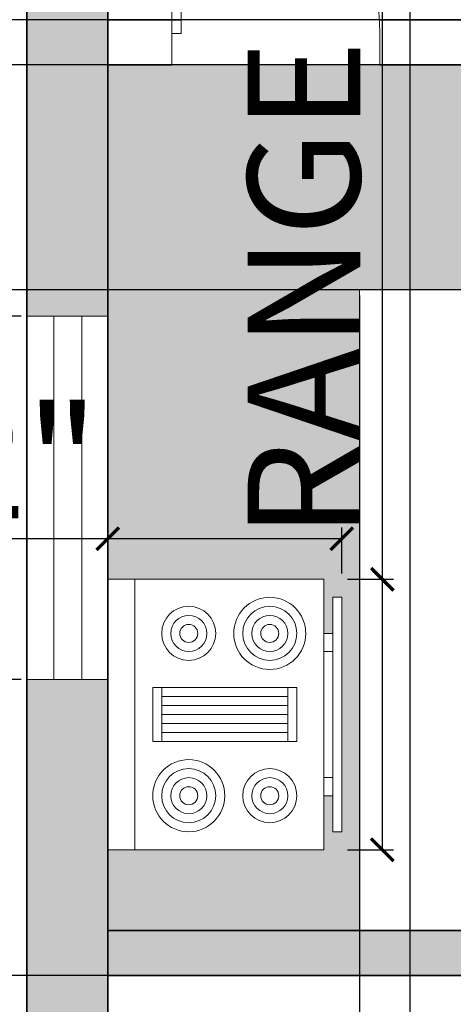
# Model space of a CAD drawing. Units: inches. Extents: x 1763 to 2368, y 1500 to 2097.
# Tile 7 of 24: x 1828 to 1876, y 1877 to 1986. Entities that reach past the tile are written whole.
import ezdxf

# ---------------------------------------------------------------- set-up
doc = ezdxf.new("R2010")
doc.units = ezdxf.units.IN
for name, color, linetype, lineweight in [('A-ANNO-DIMS', 2, 'Continuous', 18), ('A-DOOR', 4, 'Continuous', 18), ('A-EQPM', 9, 'Continuous', 18), ('A-FLOR-CASE', 8, 'Continuous', 18), ('A-WALL', 7, 'Continuous', 35), ('A-WALL-PATT', 7, 'Continuous', 13), ('windows', 1, 'Continuous', 18)]:
    doc.layers.add(name, color=color, linetype=linetype, lineweight=lineweight)
doc.layers.add('A-FLOR-CASE-PATT', color=254, linetype='Continuous', lineweight=13, true_color=0xcecce6)
doc.styles.get("Standard").update_dxf_attribs({"font": 'arial.ttf'})
doc.dimstyles.new('ISO-25', dxfattribs={"dimtxt": 12.5, "dimasz": 2.5, "dimexe": 1.25, "dimexo": 0.625, "dimtad": 1, "dimdec": 0, "dimlunit": 4, "dimtxsty": 'Standard', "dimblk": 'ARCHTICK', "dimcen": 2.5, "dimclrd": 3, "dimclrt": 4, "dimadec": 0, "dimazin": 0, "dimtfac": 1, "dimtdec": 0, "dimtmove": 0, "dimatfit": 3, "dimfxl": 1, "dimarcsym": 0})

# ---------------------------------------------------------------- blocks, each defined once
blk = doc.blocks.new('*U3')
for p, q in [((0, 0), (0, -6)), ((40, 0), (40, -6))]:
    blk.add_line(p, q)
blk.add_lwpolyline([(0, 0), (0, 40), (1.75, 40), (1.75, 0)], close=True)
blk.add_arc((0, 0), 40, 0, 90)
blk = doc.blocks.new('Range-Oven - 30 in top')
for p, q in [((0, -3), (30, -3)), ((12, -6), (18, -6)), ((13, -20), (13, -6)), ((14, -6), (14, -20)), ((15, -20), (15, -6)), ((16, -6), (16, -20)), ((17, -20), (17, -6)), ((18, -20), (12, -20)), ((6, -24), (6, -25)), ((8, -25), (8, -24)), ((22, -25), (22, -24)), ((24, -24), (24, -25))]:
    blk.add_line(p, q)
for points in [[(0, -24), (0, 0), (30, 0), (30, -24)], [(12, -21), (12, -5), (18, -5), (18, -21)], [(2, -26), (2, -25), (28, -25), (28, -26)]]:
    blk.add_lwpolyline(points, close=True)
for centre, radius in [((6, -9), 4), ((6, -9), 3), ((24, -9), 3), ((6, -9), 2), ((24, -9), 2), ((6, -9), 1), ((24, -9), 1), ((24, -18), 4), ((6, -18), 3), ((24, -18), 3), ((6, -18), 2), ((24, -18), 2), ((6, -18), 1), ((24, -18), 1)]:
    blk.add_circle(centre, radius)
blk = doc.blocks.new('_ArchTick')
at = {"color": 0, "linetype": 'ByBlock', "const_width": 0.15}
blk.add_lwpolyline([(-0.5, -0.5), (0.5, 0.5)], dxfattribs=at)
blk = doc.blocks.new('*D29')
at = {"layer": 'A-ANNO-DIMS', "color": 3, "lineweight": -2, "transparency": 16777216}
for p, q in [((1868.59, 1924.21), (1868.59, 2027.49)), ((1868.59, 1894.21), (1868.59, 1924.21))]:
    blk.add_line(p, q, dxfattribs=at)
at = {"layer": 'A-ANNO-DIMS', "color": 0, "lineweight": -2, "transparency": 16777216}
for p, q in [((1864.72, 1924.21), (1869.84, 1924.21)), ((1864.72, 1894.21), (1869.84, 1894.21))]:
    blk.add_line(p, q, dxfattribs=at)
at = {"layer": 'Defpoints', "color": 0, "transparency": 16777216}
for p in [(1864.09, 1924.21), (1868.59, 1924.21), (1864.09, 1894.21)]:
    blk.add_point(p, dxfattribs=at)
at = {"layer": 'A-ANNO-DIMS', "color": 3, "lineweight": -2, "transparency": 16777216, "xscale": 2.5, "yscale": 2.5, "zscale": 2.5}
for p, rotation in [((1868.59, 1924.21), 90), ((1868.59, 1894.21), 270)]:
    blk.add_blockref('_ArchTick', p, dxfattribs=dict(at, rotation=rotation))
at = {"layer": 'A-ANNO-DIMS', "color": 4, "transparency": 16777216, "insert": (1861.5, 1977.1), "char_height": 12.5, "attachment_point": 5, "rotation": 90}
blk.add_mtext('RANGE 2\'-6"', dxfattribs=at)
blk = doc.blocks.new('*D30')
at = {"layer": 'A-ANNO-DIMS', "color": 0, "lineweight": -2, "transparency": 16777216}
for p, q in [((1838.09, 1924.84), (1838.09, 1929.96)), ((1864.09, 1924.84), (1864.09, 1929.96))]:
    blk.add_line(p, q, dxfattribs=at)
at = {"layer": 'A-ANNO-DIMS', "color": 3, "lineweight": -2, "transparency": 16777216}
for p, q in [((1838.09, 1928.71), (1800.9, 1928.71)), ((1864.09, 1928.71), (1838.09, 1928.71))]:
    blk.add_line(p, q, dxfattribs=at)
at = {"layer": 'Defpoints', "color": 0, "transparency": 16777216}
for p in [(1838.09, 1928.71), (1838.09, 1924.21), (1864.09, 1924.21)]:
    blk.add_point(p, dxfattribs=at)
at = {"layer": 'A-ANNO-DIMS', "color": 3, "lineweight": -2, "transparency": 16777216, "xscale": 2.5, "yscale": 2.5, "zscale": 2.5, "rotation": 180}
blk.add_blockref('_ArchTick', (1838.09, 1928.71), dxfattribs=at)
at = {"layer": 'A-ANNO-DIMS', "color": 3, "lineweight": -2, "transparency": 16777216, "xscale": 2.5, "yscale": 2.5, "zscale": 2.5}
blk.add_blockref('_ArchTick', (1864.09, 1928.71), dxfattribs=at)
at = {"layer": 'A-ANNO-DIMS', "color": 4, "transparency": 16777216, "insert": (1818.25, 1935.61), "char_height": 12.5, "attachment_point": 5}
blk.add_mtext('2\'-2"', dxfattribs=at)
blk = doc.blocks.new('*D44')
at = {"layer": 'A-ANNO-DIMS', "color": 0, "lineweight": -2, "transparency": 16777216}
for p, q in [((1828.47, 2043.27), (1787.6, 2043.27)), ((1837.47, 1986.27), (1787.6, 1986.27))]:
    blk.add_line(p, q, dxfattribs=at)
at = {"layer": 'A-ANNO-DIMS', "color": 3, "lineweight": -2, "transparency": 16777216}
blk.add_line((1788.85, 2043.27), (1788.85, 1986.27), dxfattribs=at)
at = {"layer": 'Defpoints', "color": 0, "transparency": 16777216}
for p in [(1829.09, 2043.27), (1788.85, 1986.27), (1838.09, 1986.27)]:
    blk.add_point(p, dxfattribs=at)
at = {"layer": 'A-ANNO-DIMS', "color": 3, "lineweight": -2, "transparency": 16777216, "xscale": 2.5, "yscale": 2.5, "zscale": 2.5}
for p, rotation in [((1788.85, 2043.27), 90), ((1788.85, 1986.27), 270)]:
    blk.add_blockref('_ArchTick', p, dxfattribs=dict(at, rotation=rotation))
at = {"layer": 'A-ANNO-DIMS', "color": 4, "transparency": 16777216, "insert": (1781.85, 2014.77), "char_height": 12.5, "attachment_point": 5, "rotation": 90}
blk.add_mtext('4\'-9"', dxfattribs=at)
blk = doc.blocks.new('*D48')
at = {"layer": 'A-ANNO-DIMS', "color": 3, "lineweight": -2, "transparency": 16777216}
for p, q in [((1788.85, 1862.2), (1788.85, 1928.3)), ((1788.85, 1825.59), (1788.85, 1862.2))]:
    blk.add_line(p, q, dxfattribs=at)
at = {"layer": 'A-ANNO-DIMS', "color": 0, "lineweight": -2, "transparency": 16777216}
for p, q in [((1828.47, 1862.2), (1787.6, 1862.2)), ((1828.47, 1825.59), (1787.6, 1825.59))]:
    blk.add_line(p, q, dxfattribs=at)
at = {"layer": 'Defpoints', "color": 0, "transparency": 16777216}
for p in [(1788.85, 1862.2), (1829.09, 1862.2), (1829.09, 1825.59)]:
    blk.add_point(p, dxfattribs=at)
at = {"layer": 'A-ANNO-DIMS', "color": 3, "lineweight": -2, "transparency": 16777216, "xscale": 2.5, "yscale": 2.5, "zscale": 2.5}
for p, rotation in [((1788.85, 1862.2), 90), ((1788.85, 1825.59), 270)]:
    blk.add_blockref('_ArchTick', p, dxfattribs=dict(at, rotation=rotation))
at = {"layer": 'A-ANNO-DIMS', "color": 4, "transparency": 16777216, "insert": (1781.76, 1896.5), "char_height": 12.5, "attachment_point": 5, "rotation": 90}
blk.add_mtext('3\'-0 1/2"', dxfattribs=at)
blk = doc.blocks.new('*D49')
at = {"layer": 'A-ANNO-DIMS', "color": 0, "lineweight": -2, "transparency": 16777216}
for p, q in [((1828.47, 1913.1), (1787.6, 1913.1)), ((1828.47, 1862.2), (1787.6, 1862.2))]:
    blk.add_line(p, q, dxfattribs=at)
at = {"layer": 'A-ANNO-DIMS', "color": 3, "lineweight": -2, "transparency": 16777216}
blk.add_line((1788.85, 1862.2), (1788.85, 1913.1), dxfattribs=at)
at = {"layer": 'Defpoints', "color": 0, "transparency": 16777216}
for p in [(1788.85, 1913.1), (1829.09, 1913.1), (1829.09, 1862.2)]:
    blk.add_point(p, dxfattribs=at)
at = {"layer": 'A-ANNO-DIMS', "color": 3, "lineweight": -2, "transparency": 16777216, "xscale": 2.5, "yscale": 2.5, "zscale": 2.5}
for p, rotation in [((1788.85, 1913.1), 90), ((1788.85, 1862.2), 270)]:
    blk.add_blockref('_ArchTick', p, dxfattribs=dict(at, rotation=rotation))
at = {"layer": 'A-ANNO-DIMS', "color": 4, "transparency": 16777216, "insert": (1781.84, 1887.65), "char_height": 12.5, "attachment_point": 5, "rotation": 90}
blk.add_mtext('4\'-3"', dxfattribs=at)
blk = doc.blocks.new('*D50')
at = {"layer": 'A-ANNO-DIMS', "color": 3, "lineweight": -2, "transparency": 16777216}
for p, q in [((1788.85, 1953.39), (1788.85, 2019.48)), ((1788.85, 1913.1), (1788.85, 1953.39))]:
    blk.add_line(p, q, dxfattribs=at)
at = {"layer": 'A-ANNO-DIMS', "color": 0, "lineweight": -2, "transparency": 16777216}
for p, q in [((1828.47, 1953.39), (1787.6, 1953.39)), ((1828.47, 1913.1), (1787.6, 1913.1))]:
    blk.add_line(p, q, dxfattribs=at)
at = {"layer": 'Defpoints', "color": 0, "transparency": 16777216}
for p in [(1788.85, 1953.39), (1829.09, 1953.39), (1829.09, 1913.1)]:
    blk.add_point(p, dxfattribs=at)
at = {"layer": 'A-ANNO-DIMS', "color": 3, "lineweight": -2, "transparency": 16777216, "xscale": 2.5, "yscale": 2.5, "zscale": 2.5}
for p, rotation in [((1788.85, 1953.39), 90), ((1788.85, 1913.1), 270)]:
    blk.add_blockref('_ArchTick', p, dxfattribs=dict(at, rotation=rotation))
at = {"layer": 'A-ANNO-DIMS', "color": 4, "transparency": 16777216, "insert": (1781.76, 1987.69), "char_height": 12.5, "attachment_point": 5, "rotation": 90}
blk.add_mtext('3\'-4 1/2"', dxfattribs=at)
blk = doc.blocks.new('*D51')
at = {"layer": 'A-ANNO-DIMS', "color": 3, "lineweight": -2, "transparency": 16777216}
for p, q in [((1788.85, 1986.27), (1788.85, 2023.46)), ((1788.85, 1953.39), (1788.85, 1986.27))]:
    blk.add_line(p, q, dxfattribs=at)
at = {"layer": 'A-ANNO-DIMS', "color": 0, "lineweight": -2, "transparency": 16777216}
for p, q in [((1837.47, 1986.27), (1787.6, 1986.27)), ((1828.47, 1953.39), (1787.6, 1953.39))]:
    blk.add_line(p, q, dxfattribs=at)
at = {"layer": 'Defpoints', "color": 0, "transparency": 16777216}
for p in [(1788.85, 1986.27), (1838.09, 1986.27), (1829.09, 1953.39)]:
    blk.add_point(p, dxfattribs=at)
at = {"layer": 'A-ANNO-DIMS', "color": 3, "lineweight": -2, "transparency": 16777216, "xscale": 2.5, "yscale": 2.5, "zscale": 2.5}
for p, rotation in [((1788.85, 1986.27), 90), ((1788.85, 1953.39), 270)]:
    blk.add_blockref('_ArchTick', p, dxfattribs=dict(at, rotation=rotation))
at = {"layer": 'A-ANNO-DIMS', "color": 4, "transparency": 16777216, "insert": (1781.85, 2006.12), "char_height": 12.5, "attachment_point": 5, "rotation": 90}
blk.add_mtext('2\'-9"', dxfattribs=at)
blk = doc.blocks.new('*D58')
at = {"layer": 'A-ANNO-DIMS', "color": 0, "lineweight": -2, "transparency": 16777216}
for p, q in [((1871.68, 1635.9), (1871.68, 2072.02)), ((1927.07, 1635.9), (1927.07, 2072.02))]:
    blk.add_line(p, q, dxfattribs=at)
at = {"layer": 'A-ANNO-DIMS', "color": 3, "lineweight": -2, "transparency": 16777216}
for p, q in [((1871.68, 2070.77), (1927.07, 2070.77)), ((1927.07, 2070.77), (1993.68, 2070.77))]:
    blk.add_line(p, q, dxfattribs=at)
at = {"layer": 'Defpoints', "color": 0, "transparency": 16777216}
for p in [(1927.07, 2070.77), (1871.68, 1635.27), (1927.07, 1635.27)]:
    blk.add_point(p, dxfattribs=at)
at = {"layer": 'A-ANNO-DIMS', "color": 3, "lineweight": -2, "transparency": 16777216, "xscale": 2.5, "yscale": 2.5, "zscale": 2.5, "rotation": 180}
blk.add_blockref('_ArchTick', (1871.68, 2070.77), dxfattribs=at)
at = {"layer": 'A-ANNO-DIMS', "color": 3, "lineweight": -2, "transparency": 16777216, "xscale": 2.5, "yscale": 2.5, "zscale": 2.5}
blk.add_blockref('_ArchTick', (1927.07, 2070.77), dxfattribs=at)
at = {"layer": 'A-ANNO-DIMS', "color": 4, "transparency": 16777216, "insert": (1961.63, 2077.86), "char_height": 12.5, "attachment_point": 5}
blk.add_mtext('4\'-7 1/2"', dxfattribs=at)
blk = doc.blocks.new('*D69')
at = {"layer": 'A-ANNO-DIMS', "color": 0, "lineweight": -2, "transparency": 16777216}
for p, q in [((1838.09, 1879.65), (1838.09, 1509.91)), ((1895.59, 1879.65), (1895.59, 1509.91))]:
    blk.add_line(p, q, dxfattribs=at)
at = {"layer": 'A-ANNO-DIMS', "color": 3, "lineweight": -2, "transparency": 16777216}
for p, q in [((1838.09, 1511.16), (1895.59, 1511.16)), ((1895.59, 1511.16), (1962.2, 1511.16))]:
    blk.add_line(p, q, dxfattribs=at)
at = {"layer": 'Defpoints', "color": 0, "transparency": 16777216}
for p in [(1838.09, 1880.27), (1895.59, 1880.27), (1895.59, 1511.16)]:
    blk.add_point(p, dxfattribs=at)
at = {"layer": 'A-ANNO-DIMS', "color": 3, "lineweight": -2, "transparency": 16777216, "xscale": 2.5, "yscale": 2.5, "zscale": 2.5, "rotation": 180}
blk.add_blockref('_ArchTick', (1838.09, 1511.16), dxfattribs=at)
at = {"layer": 'A-ANNO-DIMS', "color": 3, "lineweight": -2, "transparency": 16777216, "xscale": 2.5, "yscale": 2.5, "zscale": 2.5}
blk.add_blockref('_ArchTick', (1895.59, 1511.16), dxfattribs=at)
at = {"layer": 'A-ANNO-DIMS', "color": 4, "transparency": 16777216, "insert": (1930.15, 1518.24), "char_height": 12.5, "attachment_point": 5}
blk.add_mtext('4\'-9 1/2"', dxfattribs=at)
blk = doc.blocks.new('*D81')
at = {"layer": 'A-ANNO-DIMS', "color": 3, "lineweight": -2, "transparency": 16777216}
for p, q in [((1788.85, 1866.87), (1788.85, 1912.38)), ((1788.85, 1843.77), (1788.85, 1866.87))]:
    blk.add_line(p, q, dxfattribs=at)
at = {"layer": 'A-ANNO-DIMS', "color": 0, "lineweight": -2, "transparency": 16777216}
for p, q in [((2077.47, 1866.87), (1787.6, 1866.87)), ((2077.47, 1843.77), (1787.6, 1843.77))]:
    blk.add_line(p, q, dxfattribs=at)
at = {"layer": 'Defpoints', "color": 0, "transparency": 16777216}
for p in [(1788.85, 1866.87), (2078.09, 1866.87), (2078.09, 1843.77)]:
    blk.add_point(p, dxfattribs=at)
at = {"layer": 'A-ANNO-DIMS', "color": 3, "lineweight": -2, "transparency": 16777216, "xscale": 2.5, "yscale": 2.5, "zscale": 2.5}
for p, rotation in [((1788.85, 1866.87), 90), ((1788.85, 1843.77), 270)]:
    blk.add_blockref('_ArchTick', p, dxfattribs=dict(at, rotation=rotation))
at = {"layer": 'A-ANNO-DIMS', "color": 4, "transparency": 16777216, "insert": (1781.95, 1890.87), "char_height": 12.5, "attachment_point": 5, "rotation": 90}
blk.add_mtext('1\'-11"', dxfattribs=at)
blk = doc.blocks.new('*D82')
at = {"layer": 'A-ANNO-DIMS', "color": 3, "lineweight": -2, "transparency": 16777216}
for p, q in [((1788.85, 1843.77), (1788.85, 1909.87)), ((1788.85, 1837.27), (1788.85, 1843.77))]:
    blk.add_line(p, q, dxfattribs=at)
at = {"layer": 'A-ANNO-DIMS', "color": 0, "lineweight": -2, "transparency": 16777216}
for p, q in [((2077.47, 1843.77), (1787.6, 1843.77)), ((2077.47, 1837.27), (1787.6, 1837.27))]:
    blk.add_line(p, q, dxfattribs=at)
at = {"layer": 'Defpoints', "color": 0, "transparency": 16777216}
for p in [(1788.85, 1843.77), (2078.09, 1843.77), (2078.09, 1837.27)]:
    blk.add_point(p, dxfattribs=at)
at = {"layer": 'A-ANNO-DIMS', "color": 3, "lineweight": -2, "transparency": 16777216, "xscale": 2.5, "yscale": 2.5, "zscale": 2.5}
for p, rotation in [((1788.85, 1843.77), 90), ((1788.85, 1837.27), 270)]:
    blk.add_blockref('_ArchTick', p, dxfattribs=dict(at, rotation=rotation))
at = {"layer": 'A-ANNO-DIMS', "color": 4, "transparency": 16777216, "insert": (1781.77, 1878.07), "char_height": 12.5, "attachment_point": 5, "rotation": 90}
blk.add_mtext('0\'-6 1/2"', dxfattribs=at)
blk = doc.blocks.new('*D85')
at = {"layer": 'A-ANNO-DIMS', "color": 0, "lineweight": -2, "transparency": 16777216}
for p, q in [((1957.47, 1986.27), (1787.6, 1986.27)), ((1958.51, 1880.27), (1787.6, 1880.27))]:
    blk.add_line(p, q, dxfattribs=at)
at = {"layer": 'A-ANNO-DIMS', "color": 3, "lineweight": -2, "transparency": 16777216}
blk.add_line((1788.85, 1986.27), (1788.85, 1880.27), dxfattribs=at)
at = {"layer": 'Defpoints', "color": 0, "transparency": 16777216}
for p in [(1958.09, 1986.27), (1788.85, 1880.27), (1959.13, 1880.27)]:
    blk.add_point(p, dxfattribs=at)
at = {"layer": 'A-ANNO-DIMS', "color": 3, "lineweight": -2, "transparency": 16777216, "xscale": 2.5, "yscale": 2.5, "zscale": 2.5}
for p, rotation in [((1788.85, 1986.27), 90), ((1788.85, 1880.27), 270)]:
    blk.add_blockref('_ArchTick', p, dxfattribs=dict(at, rotation=rotation))
at = {"layer": 'A-ANNO-DIMS', "color": 4, "transparency": 16777216, "insert": (1781.85, 1933.27), "char_height": 12.5, "attachment_point": 5, "rotation": 90}
blk.add_mtext('8\'-10"', dxfattribs=at)
blk = doc.blocks.new('*D90')
at = {"layer": 'A-ANNO-DIMS', "color": 0, "lineweight": -2, "transparency": 16777216}
for p, q in [((1838.09, 1980.65), (1838.09, 1509.91)), ((1866.04, 1955.7), (1866.04, 1509.91))]:
    blk.add_line(p, q, dxfattribs=at)
at = {"layer": 'A-ANNO-DIMS', "color": 3, "lineweight": -2, "transparency": 16777216}
for p, q in [((1838.09, 1511.16), (1866.04, 1511.16)), ((1866.04, 1511.16), (1903.23, 1511.16))]:
    blk.add_line(p, q, dxfattribs=at)
at = {"layer": 'Defpoints', "color": 0, "transparency": 16777216}
for p in [(1838.09, 1981.27), (1866.04, 1956.32), (1866.04, 1511.16)]:
    blk.add_point(p, dxfattribs=at)
at = {"layer": 'A-ANNO-DIMS', "color": 3, "lineweight": -2, "transparency": 16777216, "xscale": 2.5, "yscale": 2.5, "zscale": 2.5, "rotation": 180}
blk.add_blockref('_ArchTick', (1838.09, 1511.16), dxfattribs=at)
at = {"layer": 'A-ANNO-DIMS', "color": 3, "lineweight": -2, "transparency": 16777216, "xscale": 2.5, "yscale": 2.5, "zscale": 2.5}
blk.add_blockref('_ArchTick', (1866.04, 1511.16), dxfattribs=at)
at = {"layer": 'A-ANNO-DIMS', "color": 4, "transparency": 16777216, "insert": (1885.88, 1518.06), "char_height": 12.5, "attachment_point": 5}
blk.add_mtext('2\'-4"', dxfattribs=at)
blk = doc.blocks.new('*D91')
at = {"layer": 'A-ANNO-DIMS', "color": 0, "lineweight": -2, "transparency": 16777216}
for p, q in [((1935.72, 1981.27), (1787.6, 1981.27)), ((1935.72, 1956.32), (1787.6, 1956.32))]:
    blk.add_line(p, q, dxfattribs=at)
at = {"layer": 'A-ANNO-DIMS', "color": 3, "lineweight": -2, "transparency": 16777216}
for p, q in [((1788.85, 1981.27), (1788.85, 1956.32)), ((1788.85, 1956.32), (1788.85, 1919.13))]:
    blk.add_line(p, q, dxfattribs=at)
at = {"layer": 'Defpoints', "color": 0, "transparency": 16777216}
for p in [(1936.34, 1981.27), (1788.85, 1956.32), (1936.34, 1956.32)]:
    blk.add_point(p, dxfattribs=at)
at = {"layer": 'A-ANNO-DIMS', "color": 3, "lineweight": -2, "transparency": 16777216, "xscale": 2.5, "yscale": 2.5, "zscale": 2.5}
for p, rotation in [((1788.85, 1981.27), 90), ((1788.85, 1956.32), 270)]:
    blk.add_blockref('_ArchTick', p, dxfattribs=dict(at, rotation=rotation))
at = {"layer": 'A-ANNO-DIMS', "color": 4, "transparency": 16777216, "insert": (1781.95, 1936.48), "char_height": 12.5, "attachment_point": 5, "rotation": 90}
blk.add_mtext('2\'-1"', dxfattribs=at)

msp = doc.modelspace()

# ---------------------------------------------------------------- hatches: boundary and pattern name
at = {"layer": 'A-FLOR-CASE-PATT'}
h = msp.add_hatch(color=256, dxfattribs=at)
h.dxf.hatch_style = 1
h.paths.add_polyline_path([(1866.04, 1956.32), (1936.34, 1956.32), (1936.34, 1981.27), (1909.18, 1981.27, -0.414214), (1910.68, 1979.77), (1910.68, 1962.77, -0.414214), (1909.18, 1961.27), (1882.18, 1961.27, -0.414214), (1880.68, 1962.77), (1880.68, 1979.77, -0.414214), (1882.18, 1981.27), (1868.32, 1981.27), (1845.22, 1981.27), (1838.09, 1981.27), (1838.09, 1924.21), (1862.09, 1924.21), (1862.09, 1918.21), (1863.09, 1918.21), (1863.09, 1922.21), (1864.09, 1922.21), (1864.09, 1896.21), (1863.09, 1896.21), (1863.09, 1900.21), (1862.09, 1900.21), (1862.09, 1894.21), (1838.09, 1894.21), (1838.09, 1885.27), (1866.04, 1885.27)])
at = {"layer": 'A-WALL-PATT'}
h = msp.add_hatch(color=256, dxfattribs=at)
h.dxf.hatch_style = 1
h.paths.add_polyline_path([(1838.09, 2034.27), (1838.09, 2043.27), (1829.09, 2043.27), (1829.09, 1953.39), (1838.09, 1953.39)])
h.paths.add_polyline_path([(1838.09, 1913.1), (1829.09, 1913.1), (1829.09, 1862.2), (1838.09, 1862.2)])
h.paths.add_polyline_path([(1838.09, 1825.59), (1829.09, 1825.59), (1829.09, 1738.64), (1838.09, 1738.64)])
h.paths.add_polyline_path([(1895.59, 1885.27), (1838.09, 1885.27), (1838.09, 1880.27), (1895.59, 1880.27)])
h.paths.add_polyline_path([(1857.39, 1784.27), (1838.09, 1784.27), (1838.09, 1779.27), (1857.39, 1779.27)])
h.paths.add_polyline_path([(1958.09, 1981.27), (1971.46, 1981.27), (1971.46, 1986.27), (1968.57, 1986.27), (1958.09, 1986.27), (1953.09, 1986.27), (1927.39, 1986.27), (1927.39, 1981.27), (1953.09, 1981.27), (1953.09, 1885.27), (1932.01, 1885.27), (1932.01, 1880.27), (1959.13, 1880.27), (1959.13, 1883.74), (1959.13, 1885.27), (1958.09, 1885.27)])
h.paths.add_polyline_path([(2018.09, 1981.27), (2031.02, 1981.27), (2031.02, 1986.27), (2018.09, 1986.27), (2013.09, 1986.27), (2001.23, 1986.27), (2001.23, 1981.27), (2013.09, 1981.27), (2013.09, 1885.27), (1982.18, 1885.27, -0.016629), (1982.23, 1883.74), (1982.23, 1880.27), (2049.69, 1880.27), (2049.69, 1883.74, -0.016629), (2049.74, 1885.27), (2018.09, 1885.27)])
h.paths.add_polyline_path([(2083.09, 1981.27), (2120.61, 1981.27), (2120.61, 1986.27), (2083.09, 1986.27), (2078.09, 1986.27), (2063.14, 1986.27), (2063.14, 1981.27), (2078.09, 1981.27), (2078.09, 1885.27), (2072.78, 1885.27), (2072.78, 1883.74), (2072.78, 1880.27), (2078.09, 1880.27), (2078.09, 1866.87), (2081.56, 1866.87, -0.016629), (2083.09, 1866.82)])
h.paths.add_polyline_path([(1871.68, 1635.27), (1838.09, 1635.27), (1838.09, 1626.27), (1871.68, 1626.27)], flags=17)
h.paths.add_polyline_path([(2100.58, 1688.27), (2060.09, 1688.27), (2060.09, 1679.27), (2100.58, 1679.27)], flags=17)
h.paths.add_polyline_path([(2180.09, 1688.27), (2148.74, 1688.27), (2148.74, 1679.27), (2180.09, 1679.27)], flags=17)
h.paths.add_polyline_path([(2189.09, 1746.22), (2180.09, 1746.22), (2180.09, 1743.42), (2180.12, 1743.42), (2180.12, 1726.72), (2180.09, 1572.27), (2034.91, 1572.27), (2034.91, 1565.6), (2034.91, 1563.27), (2189.09, 1563.27)])
h.paths.add_polyline_path([(2060.09, 1802.35, -0.016629), (2058.56, 1802.3), (2055.09, 1802.3), (2055.09, 1635.27), (2042.48, 1635.27), (2042.48, 1629.74), (2042.48, 1626.27), (2055.09, 1626.27), (2055.09, 1599.27), (2040.27, 1599.27), (2040.27, 1590.27), (2060.09, 1590.27)])
h.paths.add_polyline_path([(2019.39, 1629.74, -0.060569), (2020.06, 1635.27), (1995.09, 1635.27), (1990.09, 1635.27), (1927.07, 1635.27), (1927.07, 1626.27), (1990.09, 1626.27), (1990.09, 1590.27), (1995.09, 1590.27), (2005.2, 1590.27), (2005.2, 1599.27), (1995.09, 1599.27), (1995.09, 1626.27), (2019.39, 1626.27)])
edge = h.paths.add_edge_path()
edge.add_line((2180.09, 1837.27), (2167.2, 1837.27))
edge.add_spline(control_points=[(2167.2, 1837.27), (2167.19, 1837.27), (2167.18, 1837.27), (2167.18, 1837.27)], knot_values=[168.955493, 168.955493, 168.955493, 168.955493, 169.065871, 169.065871, 169.065871, 169.065871], degree=3, periodic=0)
edge.add_spline(control_points=[(2167.18, 1837.27), (2166.56, 1837.38), (2166.33, 1846.16), (2165.71, 1846.24)], knot_values=[159.864705, 159.864705, 159.864705, 159.864705, 168.955493, 168.955493, 168.955493, 168.955493], degree=3, periodic=0)
edge.add_line((2167.12, 1837.27), (2163.16, 1837.27))
edge.add_spline(control_points=[(2163.16, 1837.27), (2163.16, 1837.27), (2163.16, 1837.27), (2163.15, 1837.27)], knot_values=[150.537172, 150.537172, 150.537172, 150.537172, 150.553797, 150.553797, 150.553797, 150.553797], degree=3, periodic=0)
edge.add_spline(control_points=[(2163.15, 1837.27), (2162.29, 1837.29), (2161.59, 1846.23), (2160.88, 1846.24)], knot_values=[141.293426, 141.293426, 141.293426, 141.293426, 150.537172, 150.537172, 150.537172, 150.537172], degree=3, periodic=0)
edge.add_line((2163.08, 1837.27), (2158.7, 1837.27))
edge.add_spline(control_points=[(2158.7, 1837.27), (2158.7, 1837.27), (2158.7, 1837.27), (2158.7, 1837.27)], knot_values=[132.033544, 132.033544, 132.033544, 132.033544, 132.049151, 132.049151, 132.049151, 132.049151], degree=3, periodic=0)
edge.add_spline(control_points=[(2158.7, 1837.27), (2157.97, 1837.29), (2157.26, 1846.23), (2156.39, 1846.24)], knot_values=[122.786021, 122.786021, 122.786021, 122.786021, 132.033544, 132.033544, 132.033544, 132.033544], degree=3, periodic=0)
edge.add_line((2158.63, 1837.27), (2153.84, 1837.27))
edge.add_spline(control_points=[(2153.84, 1837.27), (2153.83, 1837.27), (2153.82, 1837.27), (2153.82, 1837.27)], knot_values=[113.451585, 113.451585, 113.451585, 113.451585, 113.562103, 113.562103, 113.562103, 113.562103], degree=3, periodic=0)
edge.add_spline(control_points=[(2153.82, 1837.27), (2153.17, 1837.38), (2152.88, 1846.19), (2152.4, 1846.24)], knot_values=[0, 0, 0, 0, 9.081854, 9.081854, 9.081854, 9.081854], degree=3, periodic=0)
edge.add_line((2153.76, 1837.27), (2150.39, 1837.27))
edge.add_spline(control_points=[(2150.39, 1837.27), (2150.38, 1837.27), (2150.37, 1837.27), (2150.36, 1837.27)], knot_values=[95.069382, 95.069382, 95.069382, 95.069382, 95.17519, 95.17519, 95.17519, 95.17519], degree=3, periodic=0)
edge.add_spline(control_points=[(2150.36, 1837.27), (2149.49, 1837.37), (2148.42, 1846.19), (2147.59, 1846.24)], knot_values=[85.824599, 85.824599, 85.824599, 85.824599, 95.069382, 95.069382, 95.069382, 95.069382], degree=3, periodic=0)
edge.add_line((2150.29, 1837.27), (2145.43, 1837.27))
edge.add_spline(control_points=[(2145.43, 1837.27), (2145.43, 1837.27), (2145.42, 1837.27), (2145.42, 1837.27)], knot_values=[76.505559, 76.505559, 76.505559, 76.505559, 76.547811, 76.547811, 76.547811, 76.547811], degree=3, periodic=0)
edge.add_spline(control_points=[(2145.42, 1837.27), (2144.68, 1837.31), (2143.8, 1846.19), (2142.95, 1846.24)], knot_values=[67.23945, 67.23945, 67.23945, 67.23945, 76.505559, 76.505559, 76.505559, 76.505559], degree=3, periodic=0)
edge.add_line((2145.35, 1837.27), (2134.57, 1837.27))
edge.add_spline(control_points=[(2134.57, 1837.27), (2134.57, 1837.27), (2134.56, 1837.27), (2134.56, 1837.27)], knot_values=[39.001463, 39.001463, 39.001463, 39.001463, 39.045107, 39.045107, 39.045107, 39.045107], degree=3, periodic=0)
edge.add_spline(control_points=[(2134.56, 1837.27), (2133.87, 1837.31), (2133.4, 1845.85), (2132.33, 1846.24)], knot_values=[29.79778, 29.79778, 29.79778, 29.79778, 39.001463, 39.001463, 39.001463, 39.001463], degree=3, periodic=0)
edge.add_line((2134.5, 1837.27), (2128.08, 1837.27))
edge.add_spline(control_points=[(2128.08, 1837.27), (2128.03, 1837.26), (2127.98, 1837.26), (2127.93, 1837.27)], knot_values=[19.482067, 19.482067, 19.482067, 19.482067, 19.869396, 19.869396, 19.869396, 19.869396], degree=3, periodic=0)
edge.add_spline(control_points=[(2125.01, 1846.24), (2126.16, 1844.66), (2126.82, 1837.57), (2127.93, 1837.27)], knot_values=[10.389805, 10.389805, 10.389805, 10.389805, 19.482067, 19.482067, 19.482067, 19.482067], degree=3, periodic=0)
edge.add_line((2127.93, 1837.27), (2083.09, 1837.27))
edge.add_line((2083.09, 1837.27), (2083.09, 1843.77))
edge.add_line((2083.09, 1843.77), (2081.56, 1843.77))
edge.add_line((2081.56, 1843.77), (2078.09, 1843.77))
edge.add_line((2078.09, 1843.77), (2078.09, 1837.27))
edge.add_line((2078.09, 1837.27), (2055.09, 1837.27))
edge.add_line((2055.09, 1837.27), (2055.09, 1825.4))
edge.add_line((2055.09, 1825.4), (2058.56, 1825.4))
edge.add_line((2058.56, 1825.4), (2060.09, 1825.4))
edge.add_line((2060.09, 1825.4), (2060.09, 1832.27))
edge.add_line((2060.09, 1832.27), (2122.44, 1832.27))
edge.add_spline(control_points=[(2122.44, 1832.27), (2122.73, 1832.58), (2123.01, 1832.62), (2123.28, 1832.27)], knot_values=[5.972033, 5.972033, 5.972033, 5.972033, 8.057258, 8.057258, 8.057258, 8.057258], degree=3, periodic=0)
edge.add_line((2123.28, 1832.27), (2137.95, 1832.27))
edge.add_spline(control_points=[(2137.95, 1832.27), (2137.96, 1832.27), (2137.97, 1832.27), (2137.98, 1832.27)], knot_values=[53.926862, 53.926862, 53.926862, 53.926862, 54.030075, 54.030075, 54.030075, 54.030075], degree=3, periodic=0)
edge.add_spline(control_points=[(2139.72, 1825.02), (2139.28, 1825.06), (2138.67, 1832.18), (2137.98, 1832.27)], knot_values=[54.030075, 54.030075, 54.030075, 54.030075, 61.445194, 61.445194, 61.445194, 61.445194], degree=3, periodic=0)
edge.add_line((2138.05, 1832.27), (2140.96, 1832.27))
edge.add_spline(control_points=[(2140.96, 1832.27), (2140.97, 1832.27), (2140.98, 1832.27), (2140.99, 1832.27)], knot_values=[68.854182, 68.854182, 68.854182, 68.854182, 68.971237, 68.971237, 68.971237, 68.971237], degree=3, periodic=0)
edge.add_spline(control_points=[(2143.19, 1825.02), (2142.44, 1825.07), (2141.56, 1832.16), (2140.99, 1832.27)], knot_values=[68.971237, 68.971237, 68.971237, 68.971237, 76.444911, 76.444911, 76.444911, 76.444911], degree=3, periodic=0)
edge.add_line((2141.04, 1832.27), (2145.43, 1832.27))
edge.add_spline(control_points=[(2145.43, 1832.27), (2145.44, 1832.27), (2145.45, 1832.27), (2145.46, 1832.27)], knot_values=[84.039047, 84.039047, 84.039047, 84.039047, 84.124041, 84.124041, 84.124041, 84.124041], degree=3, periodic=0)
edge.add_spline(control_points=[(2148.11, 1825.02), (2147.34, 1825.02), (2146.3, 1832.19), (2145.46, 1832.27)], knot_values=[84.124041, 84.124041, 84.124041, 84.124041, 91.773891, 91.773891, 91.773891, 91.773891], degree=3, periodic=0)
edge.add_line((2145.54, 1832.27), (2150.39, 1832.27))
edge.add_spline(control_points=[(2150.39, 1832.27), (2150.42, 1832.28), (2150.45, 1832.28), (2150.47, 1832.27)], knot_values=[99.381577, 99.381577, 99.381577, 99.381577, 99.573457, 99.573457, 99.573457, 99.573457], degree=3, periodic=0)
edge.add_spline(control_points=[(2153.97, 1825.02), (2153.09, 1825.28), (2151.53, 1832.1), (2150.47, 1832.27)], knot_values=[99.573457, 99.573457, 99.573457, 99.573457, 107.218357, 107.218357, 107.218357, 107.218357], degree=3, periodic=0)
edge.add_line((2150.57, 1832.27), (2155.6, 1832.27))
edge.add_spline(control_points=[(2155.6, 1832.27), (2155.6, 1832.27), (2155.61, 1832.27), (2155.62, 1832.27)], knot_values=[114.933058, 114.933058, 114.933058, 114.933058, 115.013624, 115.013624, 115.013624, 115.013624], degree=3, periodic=0)
edge.add_spline(control_points=[(2158.28, 1825.02), (2157.4, 1825.07), (2156.25, 1832.2), (2155.62, 1832.27)], knot_values=[115.013624, 115.013624, 115.013624, 115.013624, 122.616269, 122.616269, 122.616269, 122.616269], degree=3, periodic=0)
edge.add_line((2155.68, 1832.27), (2165.19, 1832.27))
edge.add_spline(control_points=[(2165.19, 1832.27), (2165.2, 1832.27), (2165.2, 1832.27), (2165.2, 1832.27)], knot_values=[145.488477, 145.488477, 145.488477, 145.488477, 145.516379, 145.516379, 145.516379, 145.516379], degree=3, periodic=0)
edge.add_spline(control_points=[(2167.45, 1825.02), (2166.96, 1825.02), (2166.06, 1832.25), (2165.2, 1832.27)], knot_values=[145.516379, 145.516379, 145.516379, 145.516379, 153.105469, 153.105469, 153.105469, 153.105469], degree=3, periodic=0)
edge.add_line((2165.29, 1832.27), (2168.93, 1832.27))
edge.add_spline(control_points=[(2168.93, 1832.27), (2168.98, 1832.29), (2169.04, 1832.29), (2169.1, 1832.27)], knot_values=[160.517439, 160.517439, 160.517439, 160.517439, 160.939723, 160.939723, 160.939723, 160.939723], degree=3, periodic=0)
edge.add_spline(control_points=[(2171.09, 1828.64), (2170.35, 1830.37), (2169.62, 1832.09), (2169.1, 1832.27)], knot_values=[160.939723, 160.939723, 160.939723, 160.939723, 164.738835, 164.738835, 164.738835, 164.738835], degree=3, periodic=0)
edge.add_line((2169.1, 1832.27), (2180.09, 1832.27))
edge.add_line((2180.09, 1832.27), (2180.09, 1837.27))
h.paths.add_polyline_path([(2189.09, 1885.52), (2180.09, 1885.52), (2180.09, 1813.32), (2180.12, 1813.32), (2180.12, 1796.62), (2180.12, 1795.26), (2189.09, 1795.26)])
h.paths.add_polyline_path([(2180.09, 1986.27), (2166.28, 1986.27), (2166.28, 1981.27), (2180.09, 1981.27)])
h.paths.add_polyline_path([(2189.09, 2043.27), (2180.09, 2043.27), (2180.09, 2034.27), (2180.09, 1934.11), (2189.09, 1934.11)])
h.paths.add_polyline_path([(1838.09, 1681.59), (1829.09, 1681.59), (1829.09, 1563.27), (2003.86, 1563.27), (2003.86, 1565.6), (2003.86, 1572.27), (1838.09, 1572.27)])

# ---------------------------------------------------------------- linework, layer by layer
at = {"layer": 'A-FLOR-CASE'}
for p, q in [((1868.32, 1981.27), (1845.22, 1981.27)), ((1936.34, 1956.32), (1866.04, 1956.32)), ((1866.04, 1956.32), (1866.04, 1885.27))]:
    msp.add_line(p, q, dxfattribs=at)
at = {"layer": 'A-WALL'}
for p, q in [((1838.09, 1572.27), (1838.09, 2034.27)), ((1838.09, 1986.27), (1846.24, 1986.27)), ((1868.27, 1986.27), (1953.09, 1986.27)), ((1838.09, 1981.27), (1845.22, 1981.27)), ((1868.32, 1981.27), (1953.09, 1981.27)), ((1838.09, 1885.27), (1895.59, 1885.27)), ((1838.09, 1880.27), (1895.59, 1880.27))]:
    msp.add_line(p, q, dxfattribs=at)
msp.add_lwpolyline([(2003.86, 1563.27), (1829.09, 1563.27), (1829.09, 2043.27), (2189.09, 2043.27), (2189.09, 1563.27), (2034.91, 1563.27)], dxfattribs=at)
at = {"layer": 'windows'}
for p, q in [((1838.09, 1953.39), (1829.09, 1953.39)), ((1829.09, 1953.39), (1829.09, 1913.1)), ((1832.09, 1913.1), (1832.09, 1953.39)), ((1835.23, 1913.1), (1835.23, 1953.39)), ((1838.09, 1913.1), (1838.09, 1953.39)), ((1829.09, 1913.1), (1838.09, 1913.1))]:
    msp.add_line(p, q, dxfattribs=at)

# ---------------------------------------------------------------- block references
at = {"layer": 'A-DOOR', "xscale": 0.5774759422388936, "yscale": 0.5774759422388936, "zscale": 0.5774759422388936}
msp.add_blockref('*U3', (1845.22, 1984.74), dxfattribs=at)
at = {"layer": 'A-EQPM', "rotation": 90}
msp.add_blockref('Range-Oven - 30 in top', (1838.09, 1894.21), dxfattribs=at)

# ---------------------------------------------------------------- dimensions: what is measured, and where the dimension line sits
at = {"layer": 'A-ANNO-DIMS'}
for base, p1, p2, picture, middle in [((1927.07, 2070.77), (1871.68, 1635.27), (1927.07, 1635.27), '*D58', (1961.63, 2077.86)), ((1866.0388, 1511.1561), (1838.0918, 1981.2727), (1866.0388, 1956.3234), '*D90', (1885.8845, 1518.0567)), ((1895.59, 1511.16), (1838.09, 1880.27), (1895.59, 1880.27), '*D69', (1930.15, 1518.24))]:
    dim = msp.add_linear_dim(base=base, p1=p1, p2=p2, dimstyle='ISO-25', override={"dimdec": 1, "dimlfac": 1, "dimrnd": 0, "dimzin": 1, "dimdsep": 46, "dimlunit": 4, "dimfrac": 2}, dxfattribs=at)
    dim.commit()
    dim.dimension.update_dxf_attribs({"geometry": picture, "text_midpoint": middle})
for base, p1, p2, angle, picture, middle in [((1788.85, 1986.27), (1829.09, 2043.27), (1838.09, 1986.27), 90, '*D44', (1781.85, 2014.77)), ((1788.85, 1986.27), (1829.09, 1953.39), (1838.09, 1986.27), 90, '*D51', (1781.85, 2006.12)), ((1788.85, 1953.39), (1829.09, 1913.1), (1829.09, 1953.39), 90, '*D50', (1781.76, 1987.69)), ((1788.85, 1880.27), (1958.09, 1986.27), (1959.13, 1880.27), 90, '*D85', (1781.85, 1933.27)), ((1788.8549, 1956.3234), (1936.3405, 1981.2727), (1936.3405, 1956.3234), 90, '*D91', (1781.9543, 1936.4778)), ((1838.09, 1928.71), (1864.09, 1924.21), (1838.09, 1924.21), 180, '*D30', (1818.25, 1935.61)), ((1788.85, 1862.2), (1829.09, 1825.59), (1829.09, 1862.2), 90, '*D48', (1781.76, 1896.5)), ((1788.85, 1913.1), (1829.09, 1862.2), (1829.09, 1913.1), 90, '*D49', (1781.84, 1887.65)), ((1788.85, 1866.87), (2078.09, 1843.77), (2078.09, 1866.87), 90, '*D81', (1781.95, 1890.87)), ((1788.85, 1843.77), (2078.09, 1837.27), (2078.09, 1843.77), 90, '*D82', (1781.77, 1878.07))]:
    dim = msp.add_linear_dim(base=base, p1=p1, p2=p2, angle=angle, dimstyle='ISO-25', override={"dimdec": 1, "dimlfac": 1, "dimrnd": 0, "dimzin": 1, "dimdsep": 46, "dimlunit": 4, "dimfrac": 2}, dxfattribs=at)
    dim.commit()
    dim.dimension.update_dxf_attribs({"geometry": picture, "text_midpoint": middle})
dim = msp.add_linear_dim(base=(1868.59, 1924.21), p1=(1864.09, 1894.21), p2=(1864.09, 1924.21), angle=90, text='RANGE <>', dimstyle='ISO-25', override={"dimdec": 1, "dimlfac": 1, "dimrnd": 0, "dimzin": 1, "dimdsep": 46, "dimlunit": 4, "dimfrac": 2}, dxfattribs=at)
dim.commit()
dim.dimension.update_dxf_attribs({"geometry": '*D29', "text_midpoint": (1861.5, 1977.1)})

doc.saveas('drawing.dxf')
